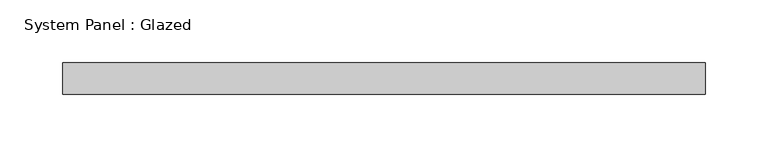
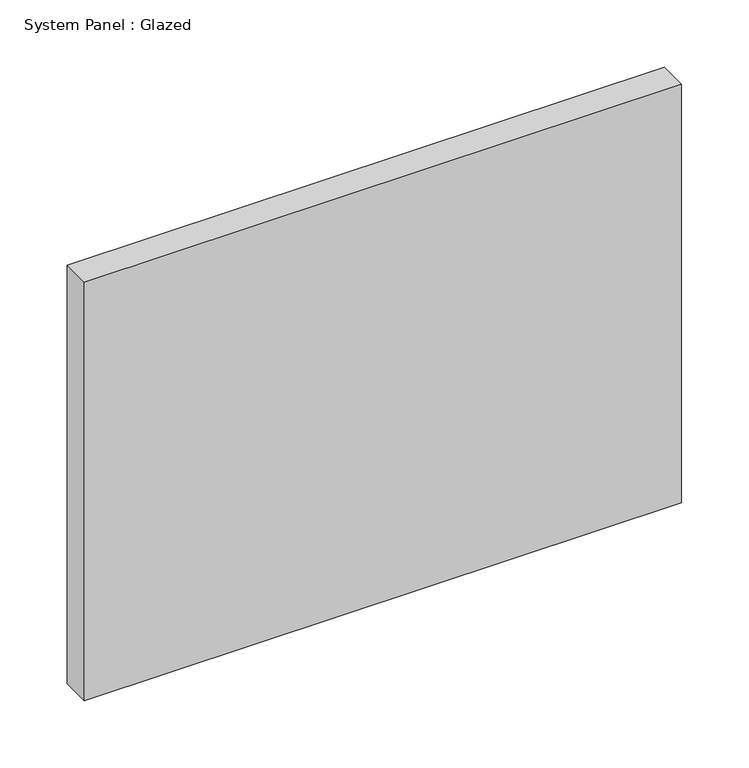
"""IFC4 building model written with IfcOpenShell, lengths in millimetres: plate geometry, System Panel : Glazed."""

from ifc_helpers import new_model, si_unit, origin, origin_with_axes, place, context, project, spatial, polyline, outline, extrude, source, transform, mapped, element, save


def system_panel_glazed_969e6b50(model_context):
    return source(origin(), model_context, "Body", "SweptSolid", [
        extrude(outline(polyline([(257.175, 19.05), (-257.175, 19.05), (-257.175, 44.45), (257.175, 44.45), (257.175, 19.05)])), origin_with_axes(), (0.0, 0.0, 1.0), 381.0),
    ])


if __name__ == "__main__":
    model = new_model("IFC4")
    model_context = context("Model", 3, world=origin())
    ifc_project = project(units=[si_unit("LENGTHUNIT", "METRE", prefix="MILLI")], contexts=[model_context])
    site = spatial("IfcSite", under=ifc_project)
    building = spatial("IfcBuilding", under=site)
    placement = place(None, origin())
    system_panel_glazed_shape = system_panel_glazed_969e6b50(model_context)
    element("IfcPlate", 1, ObjectType="System Panel : Glazed", at=placement, inside=building, context=model_context, shape_type="MappedRepresentation", body=[
        mapped(system_panel_glazed_shape, transform((0.0, 0.0, 0.0), x_axis=(1.0, 0.0, 0.0), y_axis=(0.0, 1.0, 0.0), z_axis=(0.0, 0.0, 1.0))),
    ])
    save(model, "model.ifc")

# Revit data of these elements
# Type "System Panel : Glazed"
#   Construction Type Id = "GSP4R"
#   Analytic Construction = "1/8 in Pilkington single glazing"
#   Visual Light Transmittance = 0.9
#   Solar Heat Gain Coefficient = 0.86
#   Heat Transfer Coefficient (U) = 1.18115 BTU/(h·ft²·°F)
#   Define Thermal Properties by = 1
# Element 1 (IfcPlate, "System Panel : Glazed")
#   Materials on its faces: "Glass"
# Materials
#   "Glass": class "Glass", colour RGB 0 128 192, transparency 0.75, Description = "Soda Lime Glass", Cost = 0
